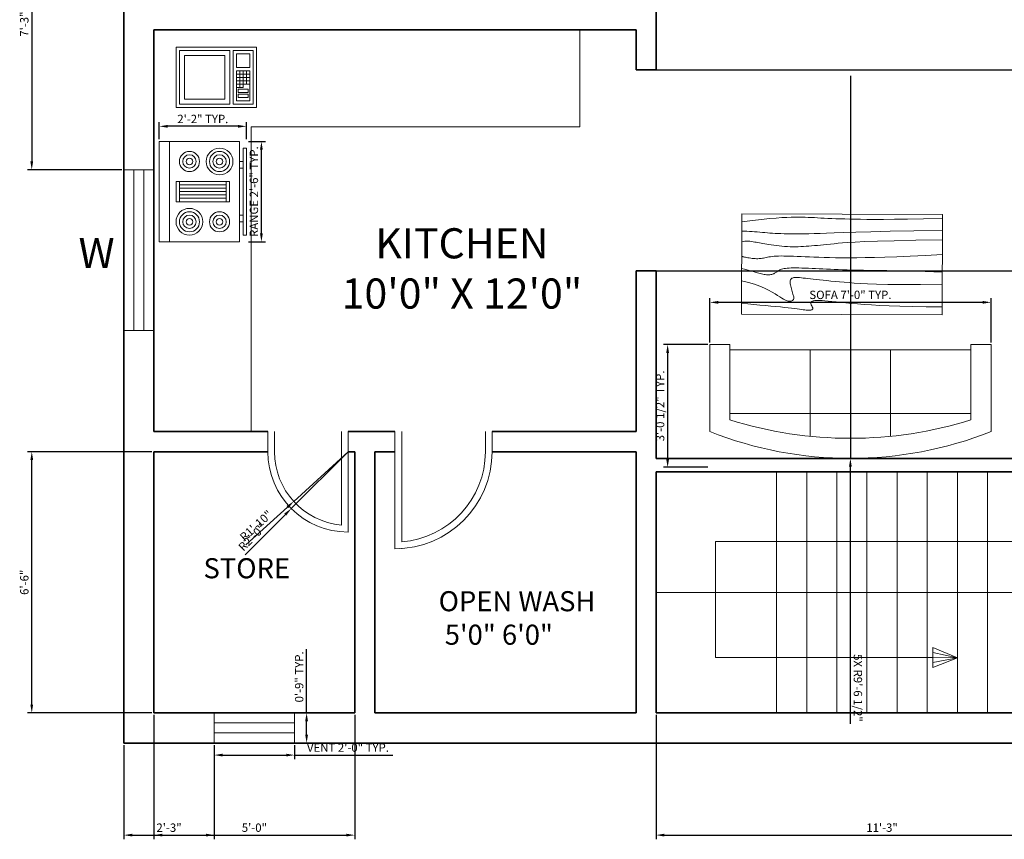
# Model space of a CAD drawing. Units: inches. Extents: x 1025 to 3479, y 1594 to 2212.
# Tile 7 of 9: x 2932 to 3226, y 1713 to 1957. Entities that reach past the tile are written whole.
import ezdxf

# ---------------------------------------------------------------- set-up
doc = ezdxf.new("R2010")
doc.units = ezdxf.units.IN
for name, color, linetype, lineweight in [('A-ANNO-DIMS', 1, 'Continuous', 18), ('A-ANNO-SYMB', 1, 'Continuous', 13), ('A-ANNO-TEXT', 7, 'Continuous', 18), ('A-AREA-IDEN', 4, 'Continuous', 18), ('A-DOOR', 4, 'Continuous', 18), ('A-EQPM', 9, 'Continuous', 18), ('A-FLOR-CSWK', 8, 'Continuous', 18), ('A-FLOR-STRS', 7, 'Continuous', 18), ('A-FURN', 8, 'Continuous', 13), ('A-GLAZ', 3, 'Continuous', 18), ('A-WALL', 7, 'Continuous', 35)]:
    doc.layers.add(name, color=color, linetype=linetype, lineweight=lineweight)
doc.styles.get("Standard").update_dxf_attribs({"font": 'arial.ttf'})
doc.dimstyles.new('ISO-25', dxfattribs={"dimtxt": 2.5, "dimasz": 2.5, "dimexe": 1.25, "dimexo": 0.625, "dimtad": 1, "dimdec": 0, "dimlunit": 3, "dimtxsty": 'Standard', "dimcen": 2.5, "dimadec": 0, "dimazin": 0, "dimtfac": 1, "dimtdec": 0, "dimtmove": 0, "dimatfit": 3, "dimfxl": 1, "dimarcsym": 0})

# ---------------------------------------------------------------- blocks, each defined once
blk = doc.blocks.new('Range-Oven - 30 in top')
for p, q in [((0, -3), (30, -3)), ((12, -6), (18, -6)), ((13, -20), (13, -6)), ((14, -6), (14, -20)), ((15, -20), (15, -6)), ((16, -6), (16, -20)), ((17, -20), (17, -6)), ((18, -20), (12, -20)), ((6, -24), (6, -25)), ((8, -25), (8, -24)), ((22, -25), (22, -24)), ((24, -24), (24, -25))]:
    blk.add_line(p, q)
for points in [[(0, -24), (0, 0), (30, 0), (30, -24)], [(12, -21), (12, -5), (18, -5), (18, -21)], [(2, -26), (2, -25), (28, -25), (28, -26)]]:
    blk.add_lwpolyline(points, close=True)
for centre, radius in [((6, -9), 4), ((6, -9), 3), ((6, -9), 2), ((6, -9), 1), ((24, -9), 3), ((24, -9), 2), ((24, -9), 1), ((24, -18), 4), ((6, -18), 3), ((6, -18), 2), ((6, -18), 1), ((24, -18), 3), ((24, -18), 2), ((24, -18), 1)]:
    blk.add_circle(centre, radius)
blk = doc.blocks.new('Microwave')
for p, q in [((18, 10), (22, 10)), ((22, 9), (18, 9)), ((19, 7), (19, 11)), ((20, 11), (20, 7)), ((21, 7), (21, 11)), ((18, 8), (22, 8)), ((22, 7), (18, 7)), ((20, 6), (18, 6)), ((19, 6), (19, 7)), ((20, 7), (20, 6))]:
    blk.add_line(p, q)
for points in [[(0, 0), (0, 18), (24, 18), (24, 0)], [(1, 1), (1, 17), (16, 17), (16, 1)], [(2.5, 2.5), (2.5, 15.5), (14.5, 15.5), (14.5, 2.5)], [(17, 1), (17, 17), (23, 17), (23, 1)], [(18, 12), (18, 16), (22, 16), (22, 12)], [(18, 2), (18, 11), (22, 11), (22, 2)], [(18.5, 4.5), (18.5, 5.5), (21.5, 5.5), (21.5, 4.5)], [(18.5, 3), (18.5, 4), (21.5, 4), (21.5, 3)]]:
    blk.add_lwpolyline(points, close=True)
blk = doc.blocks.new('Sofa - Roundback 7 ft.')
for p, q in [((-12.00002, -32.4421), (-12.00003, -6.5971)), ((11.99997, -32.4421), (11.99998, -6.5971)), ((-36.000027, -34), (-36.000027, -11.4696)), ((35.99998, -34), (35.99998, -11.4696)), ((-35.999844, -13.3819), (35.9998, -13.3819)), ((-36.000027, -32.4421), (35.99998, -32.4421))]:
    blk.add_line(p, q)
for points in [[(-36.000027, -34), (-42.000027, -34), (-42.000027, -8)], [(41.99998, -8), (41.99998, -34), (35.99998, -34)]]:
    blk.add_lwpolyline(points)
for centre, radius, start, end in [((0, -114.25), 114.25, 68.43141, 111.5686), ((-0.00001, -127.1968), 121.1968, 72.72033, 107.2797)]:
    blk.add_arc(centre, radius, start, end)
blk = doc.blocks.new('Table - Rectangular Woodgrain 60 x 30 in.')
for p, q in [((0, 0), (0, -30)), ((60, 0), (0, 0)), ((60, -30), (60, 0)), ((0, -30), (60, -30))]:
    blk.add_line(p, q)
for points in [[(0, -2.4), (4.8155, -2.418), (9.0302, -2.4688), (12.709, -2.5477), (15.9167, -2.65), (18.7181, -2.7711), (21.1781, -2.9063), (23.3616, -3.0508), (25.3333, -3.2), (27.1477, -3.3495), (28.8172, -3.4958), (30.3437, -3.636), (31.7291, -3.7667), (32.9756, -3.8849), (34.0849, -3.9875), (35.059, -4.0714), (35.9, -4.1334), (36.6114, -4.1711), (37.2041, -4.1854), (37.6906, -4.1779), (38.0833, -4.15), (38.3948, -4.1034), (38.6375, -4.0396), (38.8239, -3.9602), (38.9666, -3.8667), (39.0764, -3.7608), (39.1573, -3.6448), (39.2116, -3.521), (39.2416, -3.3917), (39.2498, -3.2593), (39.2385, -3.1261), (39.21, -2.9944), (39.1666, -2.8667), (39.111, -2.7447), (39.0468, -2.6281), (38.978, -2.5163), (38.9083, -2.4083), (38.8418, -2.3035), (38.7823, -2.201), (38.7337, -2.1001), (38.7, -2), (38.6844, -1.9003), (38.6875, -1.8021), (38.7094, -1.707), (38.75, -1.6167), (38.8094, -1.5326), (38.8875, -1.4563), (38.9844, -1.3893), (39.1, -1.3333), (39.2351, -1.2896), (39.3937, -1.2583), (39.5804, -1.2396), (39.8, -1.2333), (40.057, -1.2396), (40.3562, -1.2583), (40.7023, -1.2896), (41.1, -1.3333), (41.5547, -1.3895), (42.0755, -1.4573), (42.6721, -1.5361), (43.3542, -1.625), (44.1316, -1.7233), (45.014, -1.8302), (46.0114, -1.9449), (47.1333, -2.0667), (48.3862, -2.1947), (49.7625, -2.3281), (51.2513, -2.4663), (52.8416, -2.6083), (54.5226, -2.7535), (56.2833, -2.9011), (58.1127, -3.0501), (60, -3.2)], [(0, -9.2), (6.5759, -9.0858), (11.9385, -9.0365), (16.2527, -9.0418), (19.6833, -9.0917), (22.3952, -9.1759), (24.5531, -9.2844), (26.322, -9.4069), (27.8666, -9.5333), (29.3241, -9.6553), (30.7203, -9.7719), (32.0532, -9.8837), (33.3208, -9.9917), (34.5213, -10.0965), (35.6526, -10.199), (36.7128, -10.2999), (37.7, -10.4), (38.6129, -10.4996), (39.4531, -10.5969), (40.223, -10.6895), (40.925, -10.775), (41.5613, -10.8512), (42.1344, -10.9156), (42.6465, -10.966), (43.1, -11), (43.4976, -11.0158), (43.8437, -11.0136), (44.143, -10.9942), (44.4, -10.9583), (44.6195, -10.9069), (44.8062, -10.8406), (44.9648, -10.7603), (45.1, -10.6667), (45.2155, -10.5598), (45.3114, -10.4365), (45.3871, -10.2929), (45.4416, -10.125), (45.4743, -9.929), (45.4844, -9.7011), (45.4709, -9.4371), (45.4333, -9.1333), (45.3716, -8.7883), (45.2896, -8.4104), (45.1919, -8.0107), (45.0833, -7.6), (44.9685, -7.1893), (44.8521, -6.7896), (44.7388, -6.4117), (44.6333, -6.0667), (44.54, -5.7628), (44.4614, -5.4979), (44.4001, -5.2675), (44.3583, -5.0667), (44.3384, -4.8909), (44.3427, -4.7354), (44.3736, -4.5956), (44.4333, -4.4667), (44.5236, -4.3453), (44.6427, -4.2333), (44.7884, -4.1339), (44.9583, -4.05), (45.1501, -3.9849), (45.3614, -3.9417), (45.59, -3.9234), (45.8333, -3.9333), (46.0915, -3.9749), (46.3734, -4.0531), (46.6906, -4.1736), (47.0542, -4.3417), (47.4756, -4.5629), (47.9661, -4.8427), (48.5372, -5.1866), (49.2, -5.6), (49.9676, -6.0844), (50.8594, -6.625), (51.8965, -7.2031), (53.1, -7.8), (54.491, -8.3969), (56.0906, -8.975), (57.9199, -9.5156), (60, -10)], [(0, -12.8), (5.1847, -12.9322), (9.6213, -13.0323), (13.3963, -13.1059), (16.5958, -13.1583), (19.3063, -13.1952), (21.614, -13.2219), (23.6054, -13.2439), (25.3666, -13.2667), (26.9728, -13.2947), (28.4531, -13.3281), (29.8256, -13.3663), (31.1083, -13.4083), (32.3191, -13.4535), (33.476, -13.501), (34.597, -13.5501), (35.7, -13.6), (36.7984, -13.6497), (37.8875, -13.6979), (38.9578, -13.743), (40, -13.7833), (41.0047, -13.8174), (41.9625, -13.8438), (42.864, -13.8607), (43.7, -13.8667), (44.4631, -13.8604), (45.1552, -13.8417), (45.7801, -13.8104), (46.3416, -13.7667), (46.8439, -13.7104), (47.2906, -13.6417), (47.6858, -13.5604), (48.0333, -13.4667), (48.3375, -13.3608), (48.6042, -13.2448), (48.8396, -13.121), (49.05, -12.9917), (49.2417, -12.8593), (49.4208, -12.7261), (49.5937, -12.5944), (49.7667, -12.4667), (49.9452, -12.3451), (50.1323, -12.2313), (50.3303, -12.1268), (50.5416, -12.0333), (50.7686, -11.9524), (51.0135, -11.8854), (51.2788, -11.8341), (51.5666, -11.8), (51.8785, -11.7843), (52.2116, -11.7865), (52.562, -11.8059), (52.926, -11.8417), (53.2998, -11.8931), (53.6795, -11.9594), (54.0614, -12.0397), (54.4416, -12.1333), (54.8223, -12.2401), (55.2293, -12.3625), (55.6942, -12.5037), (56.2489, -12.6667), (56.9251, -12.8547), (57.7545, -13.0708), (58.7689, -13.3182), (60, -13.6)], [(0, -18), (5.124, -17.7273), (9.6609, -17.5057), (13.6705, -17.3303), (17.2125, -17.1958), (20.3467, -17.0973), (23.1328, -17.0297), (25.6307, -16.9878), (27.9, -16.9667), (29.9928, -16.9617), (31.9302, -16.9703), (33.7254, -16.9907), (35.3917, -17.0208), (36.9423, -17.0588), (38.3906, -17.1026), (39.7499, -17.1503), (41.0333, -17.2), (42.2519, -17.2496), (43.4073, -17.2969), (44.4986, -17.3395), (45.525, -17.375), (46.4858, -17.4012), (47.3802, -17.4156), (48.2074, -17.416), (48.9667, -17.4), (49.6583, -17.3662), (50.2872, -17.3167), (50.8595, -17.2547), (51.3812, -17.1833), (51.8584, -17.1057), (52.2971, -17.025), (52.7034, -16.9443), (53.0833, -16.8667), (53.443, -16.7951), (53.789, -16.7313), (54.128, -16.6768), (54.4666, -16.6334), (54.8115, -16.6024), (55.1693, -16.5854), (55.5465, -16.5841), (55.95, -16.6), (56.3828, -16.6337), (56.8346, -16.6823), (57.2915, -16.7418), (57.7396, -16.8084), (58.165, -16.878), (58.5539, -16.9469), (58.8924, -17.0111), (59.1666, -17.0667), (59.3679, -17.1107), (59.5078, -17.1438), (59.6032, -17.1675), (59.6708, -17.1833), (59.7275, -17.193), (59.7901, -17.1979), (59.8753, -17.1998), (60, -17.2)], [(0, -22.4), (8.0098, -22.2501), (14.4094, -22.1011), (19.4168, -21.9535), (23.25, -21.8083), (26.1269, -21.6663), (28.2656, -21.5281), (29.884, -21.3947), (31.2, -21.2667), (32.3967, -21.1448), (33.5172, -21.0292), (34.5697, -20.9198), (35.5625, -20.8167), (36.5037, -20.7198), (37.4015, -20.6292), (38.2642, -20.5448), (39.1, -20.4667), (39.9164, -20.3951), (40.7187, -20.3313), (41.5117, -20.2768), (42.3, -20.2333), (43.0883, -20.2024), (43.8812, -20.1854), (44.6836, -20.1841), (45.5, -20.2), (46.3328, -20.234), (47.1747, -20.2844), (48.0163, -20.3488), (48.8479, -20.425), (49.66, -20.5106), (50.4429, -20.6031), (51.1872, -20.7004), (51.8833, -20.8), (52.5246, -20.8999), (53.1166, -20.9995), (53.6681, -21.0983), (54.1875, -21.1958), (54.6834, -21.2919), (55.1646, -21.3859), (55.6394, -21.4777), (56.1167, -21.5667), (56.6028, -21.6515), (57.0961, -21.7266), (57.5929, -21.7852), (58.0896, -21.8208), (58.5823, -21.8268), (59.0674, -21.7964), (59.5412, -21.723), (60, -21.6)], [(0, -25.2), (8.6355, -25.0504), (15.7026, -24.9031), (21.4049, -24.7606), (25.9458, -24.625), (29.529, -24.4988), (32.3578, -24.3844), (34.6359, -24.284), (36.5667, -24.2), (38.3213, -24.1341), (39.9417, -24.0854), (41.437, -24.0523), (42.8167, -24.0333), (44.0901, -24.0268), (45.2667, -24.0313), (46.3557, -24.0451), (47.3667, -24.0667), (48.309, -24.0947), (49.1928, -24.1287), (50.0284, -24.168), (50.826, -24.2125), (51.5959, -24.2617), (52.3483, -24.3151), (53.0935, -24.3725), (53.8417, -24.4334), (54.6009, -24.497), (55.3699, -24.561), (56.1454, -24.6226), (56.9239, -24.6792), (57.7021, -24.7279), (58.4764, -24.7662), (59.2435, -24.7911), (60, -24.8)], [(0, -28.8), (5.6867, -28.6681), (10.45, -28.5698), (14.407, -28.5012), (17.675, -28.4584), (20.3711, -28.4374), (22.6125, -28.4344), (24.5164, -28.4455), (26.2, -28.4667), (27.762, -28.4947), (29.2276, -28.5281), (30.6033, -28.5663), (31.8958, -28.6084), (33.1118, -28.6535), (34.2578, -28.7011), (35.3405, -28.7501), (36.3666, -28.8), (37.3443, -28.8497), (38.288, -28.8974), (39.2137, -28.9412), (40.1375, -28.9792), (41.0753, -29.0093), (42.0432, -29.0297), (43.0572, -29.0384), (44.1333, -29.0333), (45.2936, -29.0114), (46.5843, -28.9641), (48.0579, -28.8816), (49.7666, -28.7542), (51.7629, -28.5721), (54.0989, -28.3255), (56.8272, -28.0048), (60, -27.6)]]:
    blk.add_lwpolyline(points)
blk = doc.blocks.new('WIN-48IN')
for p, q in [((0, 48), (0, 0)), ((9, 48), (0, 48)), ((3, 48), (3, 0)), ((6, 0), (6, 48)), ((9, 0), (9, 48)), ((0, 0), (9, 0))]:
    blk.add_line(p, q)
blk = doc.blocks.new('VENT-24IN')
for p, q in [((24, 9), (0, 9)), ((0, 9), (0, 0)), ((24, 0), (24, 9)), ((24, 6), (0, 6)), ((0, 3), (24, 3)), ((0, 0), (24, 0))]:
    blk.add_line(p, q)
blk = doc.blocks.new('DOOR-SWING-29IN')
for p, q in [((0, 6), (0, 35)), ((2, 6), (2, 32.93)), ((0, 6), (0, 0)), ((2, 6), (2, 0)), ((27, 0), (27, 6)), ((29, 0), (29, 6))]:
    blk.add_line(p, q)
for radius, end in [(29, 90), (27, 85.752)]:
    blk.add_arc((0, 6), radius, 0, end)
blk = doc.blocks.new('*D22')
at = {"layer": 'A-ANNO-DIMS', "color": 0, "lineweight": -2, "transparency": 16777216}
for p, q in [((2989.75, 1740.87), (2989.75, 1736.64)), ((3013.75, 1740.87), (3013.75, 1736.64)), ((2992.25, 1737.89), (3011.25, 1737.89)), ((3013.75, 1737.89), (3043.15, 1737.89))]:
    blk.add_line(p, q, dxfattribs=at)
at = {"layer": 'A-ANNO-DIMS', "color": 0, "transparency": 16777216}
for points in [[(2992.25, 1738.31), (2992.25, 1737.48), (2989.75, 1737.89)], [(3011.25, 1738.31), (3011.25, 1737.48), (3013.75, 1737.89)]]:
    blk.add_solid(points, dxfattribs=at)
at = {"layer": 'Defpoints', "color": 0, "transparency": 16777216}
for p in [(2989.75, 1741.49), (3013.75, 1741.49), (3013.75, 1737.89)]:
    blk.add_point(p, dxfattribs=at)
at = {"layer": 'A-ANNO-DIMS', "color": 0, "transparency": 16777216, "insert": (3029.7, 1739.79), "char_height": 2.5, "attachment_point": 5}
blk.add_mtext('VENT 2\'-0" TYP.', dxfattribs=at)
blk = doc.blocks.new('*D23')
at = {"layer": 'A-ANNO-DIMS', "color": 0, "lineweight": -2, "transparency": 16777216}
for p, q in [((3017.35, 1750.49), (3017.35, 1769.48)), ((3014.37, 1750.49), (3018.6, 1750.49)), ((3017.35, 1743.99), (3017.35, 1747.99)), ((3014.37, 1741.49), (3018.6, 1741.49))]:
    blk.add_line(p, q, dxfattribs=at)
at = {"layer": 'A-ANNO-DIMS', "color": 0, "transparency": 16777216}
for points in [[(3016.93, 1747.99), (3017.76, 1747.99), (3017.35, 1750.49)], [(3016.93, 1743.99), (3017.76, 1743.99), (3017.35, 1741.49)]]:
    blk.add_solid(points, dxfattribs=at)
at = {"layer": 'Defpoints', "color": 0, "transparency": 16777216}
for p in [(3013.75, 1750.49), (3017.35, 1750.49), (3013.75, 1741.49)]:
    blk.add_point(p, dxfattribs=at)
at = {"layer": 'A-ANNO-DIMS', "color": 0, "transparency": 16777216, "insert": (3015.45, 1761.24), "char_height": 2.5, "attachment_point": 5, "rotation": 90}
blk.add_mtext('0\'-9" TYP.', dxfattribs=at)
blk = doc.blocks.new('*D36')
at = {"layer": 'A-ANNO-DIMS', "color": 0, "lineweight": -2, "transparency": 16777216}
for p, q in [((3137.8, 1861.11), (3137.8, 1874.34)), ((3221.8, 1861.11), (3221.8, 1874.34)), ((3219.3, 1873.09), (3140.3, 1873.09))]:
    blk.add_line(p, q, dxfattribs=at)
at = {"layer": 'A-ANNO-DIMS', "color": 0, "transparency": 16777216}
for points in [[(3140.3, 1873.5), (3140.3, 1872.67), (3137.8, 1873.09)], [(3219.3, 1873.5), (3219.3, 1872.67), (3221.8, 1873.09)]]:
    blk.add_solid(points, dxfattribs=at)
at = {"layer": 'Defpoints', "color": 0, "transparency": 16777216}
for p in [(3137.8, 1873.09), (3137.8, 1860.49), (3221.8, 1860.49)]:
    blk.add_point(p, dxfattribs=at)
at = {"layer": 'A-ANNO-DIMS', "color": 0, "transparency": 16777216, "insert": (3179.8, 1875), "char_height": 2.5, "attachment_point": 5}
blk.add_mtext('SOFA 7\'-0" TYP.', dxfattribs=at)
blk = doc.blocks.new('*D37')
at = {"layer": 'A-ANNO-DIMS', "color": 0, "lineweight": -2, "transparency": 16777216}
for p, q in [((3137.18, 1860.49), (3123.95, 1860.49)), ((3125.2, 1857.99), (3125.2, 1826.32)), ((3137.18, 1823.82), (3123.95, 1823.82))]:
    blk.add_line(p, q, dxfattribs=at)
at = {"layer": 'A-ANNO-DIMS', "color": 0, "transparency": 16777216}
for points in [[(3124.78, 1857.99), (3125.62, 1857.99), (3125.2, 1860.49)], [(3124.78, 1826.32), (3125.62, 1826.32), (3125.2, 1823.82)]]:
    blk.add_solid(points, dxfattribs=at)
at = {"layer": 'Defpoints', "color": 0, "transparency": 16777216}
for p in [(3137.8, 1860.49), (3125.2, 1823.82), (3137.8, 1823.82)]:
    blk.add_point(p, dxfattribs=at)
at = {"layer": 'A-ANNO-DIMS', "color": 0, "transparency": 16777216, "insert": (3123.28, 1842.15), "char_height": 2.5, "attachment_point": 5, "rotation": 90}
blk.add_mtext('3\'-0 1/2" TYP.', dxfattribs=at)
blk = doc.blocks.new('*D40')
at = {"layer": 'A-ANNO-DIMS', "color": 0, "lineweight": -2, "transparency": 16777216}
for p, q in [((2999.97, 1921.15), (3005.1, 1921.15)), ((3003.85, 1893.65), (3003.85, 1918.65)), ((2999.97, 1891.15), (3005.1, 1891.15))]:
    blk.add_line(p, q, dxfattribs=at)
at = {"layer": 'A-ANNO-DIMS', "color": 0, "transparency": 16777216}
for points in [[(3003.43, 1918.65), (3004.26, 1918.65), (3003.85, 1921.15)], [(3003.43, 1893.65), (3004.26, 1893.65), (3003.85, 1891.15)]]:
    blk.add_solid(points, dxfattribs=at)
at = {"layer": 'Defpoints', "color": 0, "transparency": 16777216}
for p in [(2999.35, 1921.15), (3003.85, 1921.15), (2999.35, 1891.15)]:
    blk.add_point(p, dxfattribs=at)
at = {"layer": 'A-ANNO-DIMS', "color": 0, "transparency": 16777216, "insert": (3001.93, 1906.15), "char_height": 2.5, "attachment_point": 5, "rotation": 90}
blk.add_mtext('RANGE 2\'-6" TYP.', dxfattribs=at)
blk = doc.blocks.new('*D41')
at = {"layer": 'A-ANNO-DIMS', "color": 0, "lineweight": -2, "transparency": 16777216}
for p, q in [((2973.35, 1921.78), (2973.35, 1926.9)), ((2999.35, 1921.78), (2999.35, 1926.9)), ((2996.85, 1925.65), (2975.85, 1925.65))]:
    blk.add_line(p, q, dxfattribs=at)
at = {"layer": 'A-ANNO-DIMS', "color": 0, "transparency": 16777216}
for points in [[(2975.85, 1926.07), (2975.85, 1925.24), (2973.35, 1925.65)], [(2996.85, 1926.07), (2996.85, 1925.24), (2999.35, 1925.65)]]:
    blk.add_solid(points, dxfattribs=at)
at = {"layer": 'Defpoints', "color": 0, "transparency": 16777216}
for p in [(2973.35, 1925.65), (2973.35, 1921.15), (2999.35, 1921.15)]:
    blk.add_point(p, dxfattribs=at)
at = {"layer": 'A-ANNO-DIMS', "color": 0, "transparency": 16777216, "insert": (2986.35, 1927.53), "char_height": 2.5, "attachment_point": 5}
blk.add_mtext('2\'-2" TYP.', dxfattribs=at)
blk = doc.blocks.new('*D47')
at = {"layer": 'A-ANNO-DIMS', "color": 0, "lineweight": -2, "transparency": 16777216}
for p, q in [((2971.75, 1749.87), (2971.75, 1712.74)), ((3031.75, 1749.87), (3031.75, 1712.74)), ((2974.25, 1713.99), (3029.25, 1713.99))]:
    blk.add_line(p, q, dxfattribs=at)
at = {"layer": 'A-ANNO-DIMS', "color": 0, "transparency": 16777216}
for points in [[(2974.25, 1714.41), (2974.25, 1713.58), (2971.75, 1713.99)], [(3029.25, 1714.41), (3029.25, 1713.58), (3031.75, 1713.99)]]:
    blk.add_solid(points, dxfattribs=at)
at = {"layer": 'Defpoints', "color": 0, "transparency": 16777216}
for p in [(2971.75, 1750.49), (3031.75, 1750.49), (3031.75, 1713.99)]:
    blk.add_point(p, dxfattribs=at)
at = {"layer": 'A-ANNO-DIMS', "color": 0, "transparency": 16777216, "insert": (3001.75, 1715.89), "char_height": 2.5, "attachment_point": 5}
blk.add_mtext('5\'-0"', dxfattribs=at)
blk = doc.blocks.new('*D48')
at = {"layer": 'A-ANNO-DIMS', "color": 0, "lineweight": -2, "transparency": 16777216}
for p, q in [((2971.12, 1828.49), (2934, 1828.49)), ((2935.25, 1752.99), (2935.25, 1825.99)), ((2971.12, 1750.49), (2934, 1750.49))]:
    blk.add_line(p, q, dxfattribs=at)
at = {"layer": 'A-ANNO-DIMS', "color": 0, "transparency": 16777216}
for points in [[(2934.83, 1825.99), (2935.66, 1825.99), (2935.25, 1828.49)], [(2934.83, 1752.99), (2935.66, 1752.99), (2935.25, 1750.49)]]:
    blk.add_solid(points, dxfattribs=at)
at = {"layer": 'Defpoints', "color": 0, "transparency": 16777216}
for p in [(2935.25, 1828.49), (2971.75, 1828.49), (2971.75, 1750.49)]:
    blk.add_point(p, dxfattribs=at)
at = {"layer": 'A-ANNO-DIMS', "color": 0, "transparency": 16777216, "insert": (2933.35, 1789.49), "char_height": 2.5, "attachment_point": 5, "rotation": 90}
blk.add_mtext('6\'-6"', dxfattribs=at)
blk = doc.blocks.new('*D66')
at = {"layer": 'A-ANNO-DIMS', "color": 0, "lineweight": -2, "transparency": 16777216}
for p, q in [((2962.12, 1999.71), (2934, 1999.71)), ((2935.25, 1997.21), (2935.25, 1915.15)), ((2962.12, 1912.65), (2934, 1912.65))]:
    blk.add_line(p, q, dxfattribs=at)
at = {"layer": 'A-ANNO-DIMS', "color": 0, "transparency": 16777216}
for points in [[(2934.83, 1997.21), (2935.66, 1997.21), (2935.25, 1999.71)], [(2934.83, 1915.15), (2935.66, 1915.15), (2935.25, 1912.65)]]:
    blk.add_solid(points, dxfattribs=at)
at = {"layer": 'Defpoints', "color": 0, "transparency": 16777216}
for p in [(2962.75, 1999.71), (2935.25, 1912.65), (2962.75, 1912.65)]:
    blk.add_point(p, dxfattribs=at)
at = {"layer": 'A-ANNO-DIMS', "color": 0, "transparency": 16777216, "insert": (2933.34, 1956.18), "char_height": 2.5, "attachment_point": 5, "rotation": 90}
blk.add_mtext('7\'-3"', dxfattribs=at)
blk = doc.blocks.new('*D77')
at = {"layer": 'A-ANNO-DIMS', "color": 0, "lineweight": -2, "transparency": 16777216}
for p, q in [((2962.75, 1740.87), (2962.75, 1712.74)), ((2989.75, 1740.87), (2989.75, 1712.74)), ((2965.25, 1713.99), (2987.25, 1713.99))]:
    blk.add_line(p, q, dxfattribs=at)
at = {"layer": 'A-ANNO-DIMS', "color": 0, "transparency": 16777216}
for points in [[(2965.25, 1714.41), (2965.25, 1713.58), (2962.75, 1713.99)], [(2987.25, 1714.41), (2987.25, 1713.58), (2989.75, 1713.99)]]:
    blk.add_solid(points, dxfattribs=at)
at = {"layer": 'Defpoints', "color": 0, "transparency": 16777216}
for p in [(2962.75, 1741.49), (2989.75, 1741.49), (2989.75, 1713.99)]:
    blk.add_point(p, dxfattribs=at)
at = {"layer": 'A-ANNO-DIMS', "color": 0, "transparency": 16777216, "insert": (2976.25, 1715.89), "char_height": 2.5, "attachment_point": 5}
blk.add_mtext('2\'-3"', dxfattribs=at)
blk = doc.blocks.new('*D82')
at = {"layer": 'A-ANNO-DIMS', "color": 0, "lineweight": -2, "transparency": 16777216}
for p, q in [((3121.75, 1749.87), (3121.75, 1712.74)), ((3256.75, 1749.87), (3256.75, 1712.74)), ((3124.25, 1713.99), (3254.25, 1713.99))]:
    blk.add_line(p, q, dxfattribs=at)
at = {"layer": 'A-ANNO-DIMS', "color": 0, "transparency": 16777216}
for points in [[(3124.25, 1714.41), (3124.25, 1713.58), (3121.75, 1713.99)], [(3254.25, 1714.41), (3254.25, 1713.58), (3256.75, 1713.99)]]:
    blk.add_solid(points, dxfattribs=at)
at = {"layer": 'Defpoints', "color": 0, "transparency": 16777216}
for p in [(3121.75, 1750.49), (3256.75, 1750.49), (3256.75, 1713.99)]:
    blk.add_point(p, dxfattribs=at)
at = {"layer": 'A-ANNO-DIMS', "color": 0, "transparency": 16777216, "insert": (3189.25, 1715.89), "char_height": 2.5, "attachment_point": 5}
blk.add_mtext('11\'-3"', dxfattribs=at)
blk = doc.blocks.new('*D85')
at = {"layer": 'A-ANNO-DIMS', "color": 0, "lineweight": -2, "transparency": 16777216}
for p, q in [((3116.37, 1942.49), (3471.57, 1942.49)), ((3470.32, 1884.99), (3470.32, 1939.99)), ((3116.37, 1882.49), (3471.57, 1882.49))]:
    blk.add_line(p, q, dxfattribs=at)
at = {"layer": 'A-ANNO-DIMS', "color": 0, "transparency": 16777216}
for points in [[(3469.91, 1939.99), (3470.74, 1939.99), (3470.32, 1942.49)], [(3469.91, 1884.99), (3470.74, 1884.99), (3470.32, 1882.49)]]:
    blk.add_solid(points, dxfattribs=at)
at = {"layer": 'Defpoints', "color": 0, "transparency": 16777216}
for p in [(3115.75, 1942.49), (3470.32, 1942.49), (3115.75, 1882.49)]:
    blk.add_point(p, dxfattribs=at)
at = {"layer": 'A-ANNO-DIMS', "color": 0, "transparency": 16777216, "insert": (3468.42, 1912.49), "char_height": 2.5, "attachment_point": 5, "rotation": 90}
blk.add_mtext('5\'-0"', dxfattribs=at)
blk = doc.blocks.new('*D88')
at = {"layer": 'A-ANNO-DIMS', "color": 0, "lineweight": -2, "transparency": 16777216}
for p, q in [((3029.75, 1828.49), (3012.78, 1811.52)), ((2998.96, 1797.7), (3011.01, 1809.75))]:
    blk.add_line(p, q, dxfattribs=at)
at = {"layer": 'A-ANNO-DIMS', "color": 0, "transparency": 16777216}
blk.add_solid([(3010.71, 1810.05), (3011.3, 1809.46), (3012.78, 1811.52)], dxfattribs=at)
at = {"layer": 'Defpoints', "color": 0, "transparency": 16777216}
for p in [(3029.75, 1828.49), (3012.78, 1811.52)]:
    blk.add_point(p, dxfattribs=at)
at = {"layer": 'A-ANNO-DIMS', "color": 0, "transparency": 16777216, "insert": (3001.25, 1802.68), "char_height": 2.5, "attachment_point": 5, "rotation": 45.0001}
blk.add_mtext('R2\'-0"', dxfattribs=at)
blk = doc.blocks.new('*D91')
at = {"layer": 'A-ANNO-DIMS', "color": 0, "lineweight": -2, "transparency": 16777216}
for p, q in [((3179.8, 1940.74), (3179.8, 1826.49)), ((3179.8, 1747.19), (3179.8, 1823.99))]:
    blk.add_line(p, q, dxfattribs=at)
at = {"layer": 'A-ANNO-DIMS', "color": 0, "transparency": 16777216}
blk.add_solid([(3180.22, 1823.99), (3179.38, 1823.99), (3179.8, 1826.49)], dxfattribs=at)
at = {"layer": 'Defpoints', "color": 0, "transparency": 16777216}
for p in [(3179.8, 1940.74), (3179.8, 1826.49)]:
    blk.add_point(p, dxfattribs=at)
at = {"layer": 'A-ANNO-DIMS', "color": 0, "transparency": 16777216, "insert": (3181.72, 1757.94), "char_height": 2.5, "attachment_point": 5, "rotation": 270.0001}
blk.add_mtext('5X R9\'-6 1/2"', dxfattribs=at)
blk = doc.blocks.new('*D97')
at = {"layer": 'A-ANNO-DIMS', "color": 0, "lineweight": -2, "transparency": 16777216}
for p, q in [((3029.75, 1828.49), (3013.5, 1813.66)), ((2999.23, 1800.64), (3011.65, 1811.97))]:
    blk.add_line(p, q, dxfattribs=at)
at = {"layer": 'A-ANNO-DIMS', "color": 0, "transparency": 16777216}
blk.add_solid([(3011.37, 1812.28), (3011.93, 1811.67), (3013.5, 1813.66)], dxfattribs=at)
at = {"layer": 'Defpoints', "color": 0, "transparency": 16777216}
for p in [(3029.75, 1828.49), (3013.5, 1813.66)]:
    blk.add_point(p, dxfattribs=at)
at = {"layer": 'A-ANNO-DIMS', "color": 0, "transparency": 16777216, "insert": (3002.47, 1806.16), "char_height": 2.5, "attachment_point": 5, "rotation": 42.3934}
blk.add_mtext('R1\'-10"', dxfattribs=at)

msp = doc.modelspace()

# ---------------------------------------------------------------- linework, layer by layer
at = {"layer": 'A-ANNO-SYMB'}
for p, q in [((3241.46, 1801.64), (3139.54, 1801.64)), ((3139.54, 1801.64), (3139.54, 1767.01)), ((3204.46, 1767.01), (3204.46, 1770.01)), ((3204.46, 1770.01), (3204.46, 1767.01)), ((3211.75, 1766.93), (3204.46, 1770.01)), ((3204.46, 1770.01), (3211.75, 1766.93)), ((3204.46, 1767.01), (3204.46, 1768.51)), ((3204.46, 1768.51), (3211.75, 1766.93)), ((3139.54, 1767.01), (3204.46, 1767.01)), ((3204.46, 1767.01), (3204.46, 1764.01)), ((3211.75, 1766.93), (3204.46, 1767.01)), ((3204.46, 1764.01), (3211.75, 1766.93)), ((3211.75, 1766.93), (3204.46, 1765.51))]:
    msp.add_line(p, q, dxfattribs=at)
at = {"layer": 'A-DOOR'}
for p, q in [((3005.75, 1834.49), (3005.75, 1828.49)), ((3007.75, 1834.49), (3007.75, 1828.49)), ((3027.75, 1828.49), (3027.75, 1834.49)), ((3029.75, 1828.49), (3029.75, 1834.49)), ((3027.75, 1828.49), (3027.75, 1806.58)), ((3029.75, 1828.49), (3029.75, 1804.49)), ((3045.75, 1799.56), (3045.75, 1799.49))]:
    msp.add_line(p, q, dxfattribs=at)
for radius, end in [(24, 270), (22, 264.7841)]:
    msp.add_arc((3029.75, 1828.49), radius, 180, end, dxfattribs=at)
at = {"layer": 'A-FLOR-CSWK'}
for p, q in [((3098.93, 1954.49), (3098.93, 1925.49)), ((3000.75, 1925.49), (3098.93, 1925.49)), ((3000.75, 1834.49), (3000.75, 1925.49))]:
    msp.add_line(p, q, dxfattribs=at)
at = {"layer": 'A-FLOR-STRS'}
for p, q in [((3157.75, 1817.49), (3157.75, 1822.49)), ((3157.75, 1822.49), (3157.75, 1750.49)), ((3166.75, 1822.49), (3166.75, 1750.49)), ((3175.75, 1822.49), (3175.75, 1750.49)), ((3184.75, 1822.49), (3184.75, 1750.49)), ((3193.75, 1822.49), (3193.75, 1750.49)), ((3202.75, 1822.49), (3202.75, 1750.49)), ((3211.75, 1822.49), (3211.75, 1750.49)), ((3220.75, 1822.49), (3220.75, 1750.49)), ((3157.75, 1750.49), (3157.75, 1817.49)), ((3121.75, 1786.49), (3283.75, 1786.49))]:
    msp.add_line(p, q, dxfattribs=at)
at = {"layer": 'A-WALL'}
for p, q in [((2962.75, 1741.49), (2962.75, 2101.49)), ((3121.75, 1942.49), (3121.75, 1972.49)), ((2971.75, 1954.49), (3115.75, 1954.49)), ((2971.75, 1834.49), (2971.75, 1954.49)), ((3115.75, 1954.49), (3115.75, 1942.49)), ((3115.75, 1942.49), (3115.75, 1954.49)), ((3115.75, 1942.49), (3121.75, 1942.49)), ((3115.75, 1834.49), (3115.75, 1882.49)), ((3121.75, 1882.49), (3115.75, 1882.49)), ((3121.75, 1826.49), (3121.75, 1882.49)), ((2971.75, 1834.49), (2977.75, 1834.49)), ((2977.75, 1834.49), (3005.75, 1834.49)), ((3029.75, 1834.49), (3043.75, 1834.49)), ((3072.75, 1834.49), (3115.75, 1834.49)), ((2971.75, 1750.49), (2971.75, 1828.49)), ((2971.75, 1828.49), (2977.75, 1828.49)), ((2971.75, 1828.49), (2977.75, 1828.49)), ((3005.75, 1828.49), (2977.75, 1828.49)), ((3029.75, 1828.49), (3031.75, 1828.49)), ((3031.75, 1828.49), (3029.75, 1828.49)), ((3031.75, 1750.49), (3031.75, 1828.49)), ((3037.75, 1750.49), (3037.75, 1828.49)), ((3037.75, 1828.49), (3043.75, 1828.49)), ((3037.75, 1828.49), (3043.75, 1828.49)), ((3072.75, 1828.49), (3115.75, 1828.49)), ((3115.75, 1750.49), (3115.75, 1828.49)), ((3121.75, 1826.49), (3283.75, 1826.49)), ((3121.75, 1822.49), (3283.75, 1822.49)), ((3121.75, 1822.49), (3121.75, 1817.49)), ((3121.75, 1750.49), (3121.75, 1817.49)), ((3031.75, 1750.49), (2971.75, 1750.49)), ((3115.75, 1750.49), (3037.75, 1750.49)), ((3433.75, 1750.49), (3121.75, 1750.49)), ((3442.75, 1741.49), (2962.75, 1741.49))]:
    msp.add_line(p, q, dxfattribs=at)

# ---------------------------------------------------------------- block references
at = {"layer": 'A-DOOR', "extrusion": (0, 0, -1), "zscale": -1, "rotation": 180}
msp.add_blockref('DOOR-SWING-29IN', (-3043.75, 1834.49), dxfattribs=at)
at = {"layer": 'A-EQPM'}
msp.add_blockref('Microwave', (2978.41, 1931.26), dxfattribs=at)
at = {"layer": 'A-EQPM', "rotation": 89.99999999999999}
msp.add_blockref('Range-Oven - 30 in top', (2973.35, 1891.15), dxfattribs=at)
at = {"layer": 'A-FURN'}
for name, p, rotation in [('Table - Rectangular Woodgrain 60 x 30 in.', (3207.25, 1869.35), 179.8036337053011), ('Sofa - Roundback 7 ft.', (3179.8, 1826.49), 180)]:
    msp.add_blockref(name, p, dxfattribs=dict(at, rotation=rotation))
at = {"layer": 'A-GLAZ'}
for name, p in [('WIN-48IN', (2962.75, 1864.65)), ('VENT-24IN', (2989.75, 1741.49))]:
    msp.add_blockref(name, p, dxfattribs=at)

# ---------------------------------------------------------------- texts
at = {"layer": 'A-ANNO-TEXT', "insert": (2946.67, 1892.3), "char_height": 9, "attachment_point": 1}
msp.add_mtext_dynamic_manual_height_columns('\\pxqc;W', width=15.8719, gutter_width=12.5, heights=[0], dxfattribs=at)
at = {"layer": 'A-AREA-IDEN', "attachment_point": 1}
for s, width, insert, char_height in [('\\pxqc;KITCHEN \\P10\'0" X 12\'0"', 93.2353, (3017.14, 1895.22), 9), ('\\pxqc;STORE', 43.2814, (2977.84, 1796.68), 6), ('OPEN WASH\\P 5\'0" 6\'0"', 70.8251, (3056.79, 1786.84), 6)]:
    msp.add_mtext_dynamic_manual_height_columns(s, width=width, gutter_width=12.5, heights=[0], dxfattribs=dict(at, insert=insert, char_height=char_height))

# ---------------------------------------------------------------- dimensions: what is measured, and where the dimension line sits
at = {"layer": 'A-ANNO-DIMS'}
for base, p1, p2, picture, middle in [((2935.25, 1912.65), (2962.75, 1999.71), (2962.75, 1912.65), '*D66', (2933.34, 1956.18)), ((3470.32, 1942.49), (3115.75, 1882.49), (3115.75, 1942.49), '*D85', (3468.42, 1912.49)), ((2935.25, 1828.49), (2971.75, 1750.49), (2971.75, 1828.49), '*D48', (2933.35, 1789.49))]:
    dim = msp.add_linear_dim(base=base, p1=p1, p2=p2, angle=90, dimstyle='ISO-25', override={"dimdec": 1, "dimlfac": 1, "dimrnd": 0, "dimzin": 1, "dimdsep": 46, "dimlunit": 4, "dimfrac": 2}, dxfattribs=at)
    dim.commit()
    dim.dimension.update_dxf_attribs({"geometry": picture, "text_midpoint": middle})
dim = msp.add_radius_dim(center=(3179.800812, 1940.735859), mpoint=(3179.801, 1826.485859), text='5X <>', dimstyle='ISO-25', override={"dimdec": 1, "dimlfac": 1, "dimrnd": 0, "dimzin": 1, "dimdsep": 46, "dimlunit": 4, "dimfrac": 2}, dxfattribs=at)
dim.commit()
dim.dimension.update_dxf_attribs({"geometry": '*D91', "text_midpoint": (3179.8011128, 1757.935859), "dimtype": 164})
for base, p1, p2, angle, text, picture, middle in [((2973.35, 1925.65), (2999.35, 1921.15), (2973.35, 1921.15), 180, '<> TYP.', '*D41', (2986.35, 1927.53)), ((3003.85, 1921.15), (2999.35, 1891.15), (2999.35, 1921.15), 90, 'RANGE <> TYP.', '*D40', (3001.93, 1906.15)), ((3137.8, 1873.09), (3221.8, 1860.49), (3137.8, 1860.49), 180, 'SOFA <> TYP.', '*D36', (3179.8, 1875)), ((3125.2, 1823.82), (3137.8, 1860.49), (3137.8, 1823.82), 270, '<> TYP.', '*D37', (3123.28, 1842.15)), ((3017.35, 1750.49), (3013.75, 1741.49), (3013.75, 1750.49), 90, '<> TYP.', '*D23', (3015.45, 1761.24))]:
    dim = msp.add_linear_dim(base=base, p1=p1, p2=p2, angle=angle, text=text, dimstyle='ISO-25', override={"dimdec": 1, "dimlfac": 1, "dimrnd": 0, "dimzin": 1, "dimdsep": 46, "dimlunit": 4, "dimfrac": 2}, dxfattribs=at)
    dim.commit()
    dim.dimension.update_dxf_attribs({"geometry": picture, "text_midpoint": middle})
for mpoint, picture, middle in [((3012.78, 1811.52), '*D88', (3002.59, 1801.34)), ((3013.5, 1813.66), '*D97', (3003.75, 1804.76))]:
    dim = msp.add_radius_dim(center=(3029.75, 1828.49), mpoint=mpoint, dimstyle='ISO-25', override={"dimdec": 1, "dimlfac": 1, "dimrnd": 0, "dimzin": 1, "dimdsep": 46, "dimlunit": 4, "dimfrac": 2}, dxfattribs=at)
    dim.commit()
    dim.dimension.update_dxf_attribs({"geometry": picture, "text_midpoint": middle, "dimtype": 164})
for base, p1, p2, picture, middle in [((3031.75, 1713.99), (2971.75, 1750.49), (3031.75, 1750.49), '*D47', (3001.75, 1715.89)), ((3256.75, 1713.99), (3121.75, 1750.49), (3256.75, 1750.49), '*D82', (3189.25, 1715.89)), ((2989.75, 1713.99), (2962.75, 1741.49), (2989.75, 1741.49), '*D77', (2976.25, 1715.89))]:
    dim = msp.add_linear_dim(base=base, p1=p1, p2=p2, dimstyle='ISO-25', override={"dimdec": 1, "dimlfac": 1, "dimrnd": 0, "dimzin": 1, "dimdsep": 46, "dimlunit": 4, "dimfrac": 2}, dxfattribs=at)
    dim.commit()
    dim.dimension.update_dxf_attribs({"geometry": picture, "text_midpoint": middle})
dim = msp.add_linear_dim(base=(3013.75, 1737.89), p1=(2989.75, 1741.49), p2=(3013.75, 1741.49), text='VENT <> TYP.', dimstyle='ISO-25', override={"dimdec": 1, "dimlfac": 1, "dimrnd": 0, "dimzin": 1, "dimdsep": 46, "dimlunit": 4, "dimfrac": 2}, dxfattribs=at)
dim.commit()
dim.dimension.update_dxf_attribs({"geometry": '*D22', "text_midpoint": (3029.7, 1739.79)})

doc.saveas('drawing.dxf')
